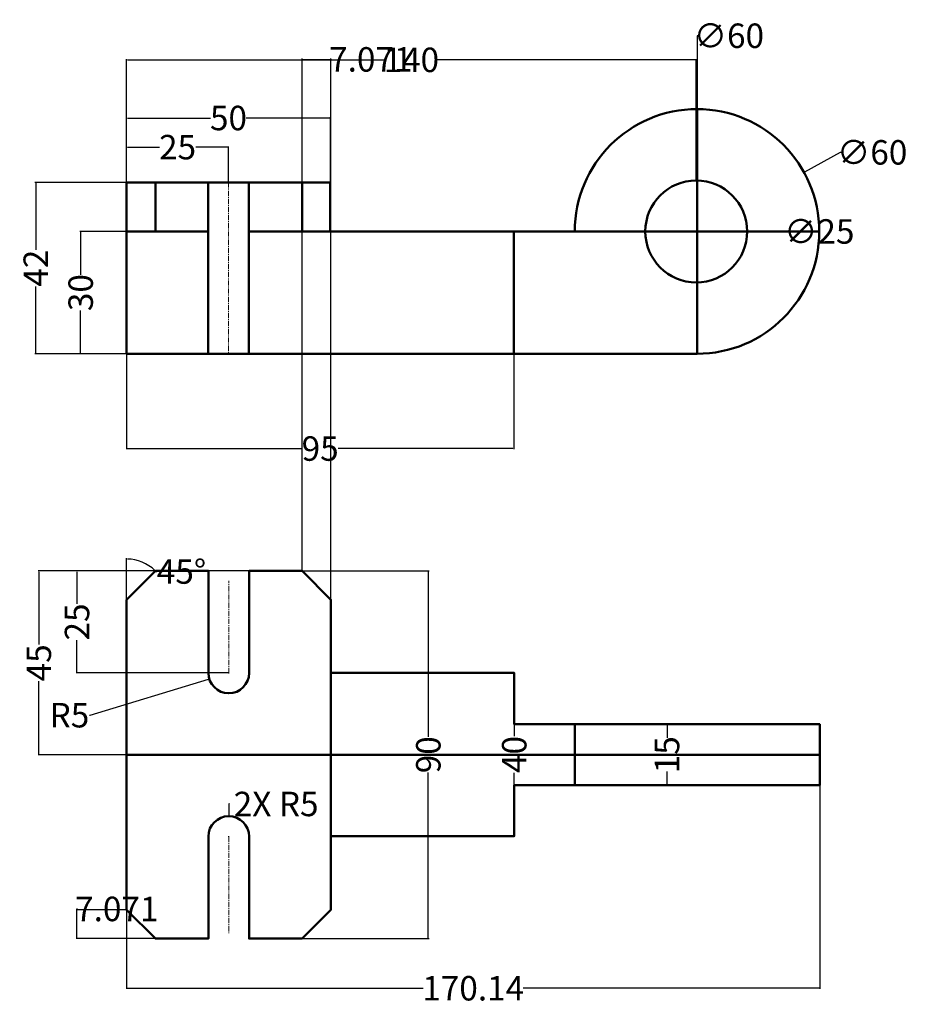
# Model space of a CAD drawing. Units: millimetres. Extents: x 4 to 222, y -16 to 226.
import ezdxf

# ---------------------------------------------------------------- set-up
doc = ezdxf.new("R2010")
doc.units = ezdxf.units.MM
doc.header["$MEASUREMENT"] = 0
doc.linetypes.add('CENTER', pattern=[2, 1.25, -0.25, 0.25, -0.25])
for name, color, linetype, lineweight in [('M-CNTR', 4, 'CENTER', 18), ('M-DIMS', 2, 'Continuous', 25), ('M-OUTL', 7, 'Continuous', 50)]:
    doc.layers.add(name, color=color, linetype=linetype, lineweight=lineweight)
doc.styles.get("Standard").update_dxf_attribs({"font": 'arial.ttf'})
doc.dimstyles.get("Standard").update_dxf_attribs({"dimtxt": 6, "dimasz": 0.18, "dimexe": 0.18, "dimexo": 0.0625, "dimgap": 0.09, "dimtad": 0, "dimtoh": 1, "dimdec": 0, "dimzin": 0, "dimdsep": 46, "dimtxsty": 'Standard', "dimcen": 0.09, "dimadec": 0, "dimazin": 0, "dimtfac": 1, "dimtdec": 0, "dimtofl": 0, "dimtmove": 0, "dimatfit": 3, "dimfxl": 1, "dimtolj": 1, "dimtzin": 0, "dimarcsym": 0})

# ---------------------------------------------------------------- blocks, each defined once
blk = doc.blocks.new('*D1')
at = {"layer": 'Defpoints', "color": 0, "transparency": 16777216}
for p in [(170.41, 216.06), (30.64, 185.97), (170.41, 186.47)]:
    blk.add_point(p, dxfattribs=at)
at = {"layer": 'M-DIMS', "color": 0, "lineweight": -2, "transparency": 16777216}
for p, q in [((30.64, 186.03), (30.64, 216.24)), ((30.82, 216.06), (94.1, 216.06)), ((170.23, 216.06), (106.95, 216.06)), ((170.41, 186.53), (170.41, 216.24))]:
    blk.add_line(p, q, dxfattribs=at)
at = {"layer": 'M-DIMS', "color": 0, "transparency": 16777216}
for points in [[(30.82, 216.09), (30.82, 216.03), (30.64, 216.06)], [(170.23, 216.09), (170.23, 216.03), (170.41, 216.06)]]:
    blk.add_solid(points, dxfattribs=at)
at = {"layer": 'M-DIMS', "color": 0, "transparency": 16777216, "insert": (100.52, 216.06), "char_height": 6, "attachment_point": 5}
blk.add_mtext('\\A1;140', dxfattribs=at)
blk = doc.blocks.new('*D2')
at = {"layer": 'Defpoints', "color": 0, "transparency": 16777216}
for p in [(80.64, 201.79), (30.64, 185.97), (80.64, 185.97)]:
    blk.add_point(p, dxfattribs=at)
at = {"layer": 'M-DIMS', "color": 0, "lineweight": -2, "transparency": 16777216}
for p, q in [((30.64, 186.03), (30.64, 201.97)), ((30.82, 201.79), (51.26, 201.79)), ((80.46, 201.79), (60.02, 201.79)), ((80.64, 186.03), (80.64, 201.97))]:
    blk.add_line(p, q, dxfattribs=at)
at = {"layer": 'M-DIMS', "color": 0, "transparency": 16777216}
for points in [[(30.82, 201.82), (30.82, 201.76), (30.64, 201.79)], [(80.46, 201.82), (80.46, 201.76), (80.64, 201.79)]]:
    blk.add_solid(points, dxfattribs=at)
at = {"layer": 'M-DIMS', "color": 0, "transparency": 16777216, "insert": (55.64, 201.79), "char_height": 6, "attachment_point": 5}
blk.add_mtext('\\A1;50', dxfattribs=at)
blk = doc.blocks.new('*D3')
at = {"layer": 'Defpoints', "color": 0, "transparency": 16777216}
for p in [(55.64, 194.65), (30.64, 185.97), (55.64, 185.97)]:
    blk.add_point(p, dxfattribs=at)
at = {"layer": 'M-DIMS', "color": 0, "lineweight": -2, "transparency": 16777216}
for p, q in [((30.64, 186.03), (30.64, 194.83)), ((30.82, 194.65), (38.68, 194.65)), ((55.46, 194.65), (47.6, 194.65)), ((55.64, 186.03), (55.64, 194.83))]:
    blk.add_line(p, q, dxfattribs=at)
at = {"layer": 'M-DIMS', "color": 0, "transparency": 16777216}
for points in [[(30.82, 194.68), (30.82, 194.62), (30.64, 194.65)], [(55.46, 194.68), (55.46, 194.62), (55.64, 194.65)]]:
    blk.add_solid(points, dxfattribs=at)
at = {"layer": 'M-DIMS', "color": 0, "transparency": 16777216, "insert": (43.14, 194.65), "char_height": 6, "attachment_point": 5}
blk.add_mtext('\\A1;25', dxfattribs=at)
blk = doc.blocks.new('*D4')
at = {"layer": 'Defpoints', "color": 0, "transparency": 16777216}
for p in [(30.64, 185.97), (8.33, 143.97), (30.64, 143.97)]:
    blk.add_point(p, dxfattribs=at)
at = {"layer": 'M-DIMS', "color": 0, "lineweight": -2, "transparency": 16777216}
for p, q in [((30.58, 185.97), (8.15, 185.97)), ((8.33, 185.79), (8.33, 169.45)), ((8.33, 144.15), (8.33, 160.49)), ((30.58, 143.97), (8.15, 143.97))]:
    blk.add_line(p, q, dxfattribs=at)
at = {"layer": 'M-DIMS', "color": 0, "transparency": 16777216}
for points in [[(8.3, 185.79), (8.36, 185.79), (8.33, 185.97)], [(8.3, 144.15), (8.36, 144.15), (8.33, 143.97)]]:
    blk.add_solid(points, dxfattribs=at)
at = {"layer": 'M-DIMS', "color": 0, "transparency": 16777216, "insert": (8.33, 164.97), "char_height": 6, "attachment_point": 5, "rotation": 90}
blk.add_mtext('\\A1;42', dxfattribs=at)
blk = doc.blocks.new('*D5')
at = {"layer": 'Defpoints', "color": 0, "transparency": 16777216}
for p in [(30.64, 173.97), (19.36, 143.97), (30.64, 143.97)]:
    blk.add_point(p, dxfattribs=at)
at = {"layer": 'M-DIMS', "color": 0, "lineweight": -2, "transparency": 16777216}
for p, q in [((30.58, 173.97), (19.18, 173.97)), ((19.36, 173.79), (19.36, 163.34)), ((19.36, 144.15), (19.36, 154.59)), ((30.58, 143.97), (19.18, 143.97))]:
    blk.add_line(p, q, dxfattribs=at)
at = {"layer": 'M-DIMS', "color": 0, "transparency": 16777216}
for points in [[(19.33, 173.79), (19.39, 173.79), (19.36, 173.97)], [(19.33, 144.15), (19.39, 144.15), (19.36, 143.97)]]:
    blk.add_solid(points, dxfattribs=at)
at = {"layer": 'M-DIMS', "color": 0, "transparency": 16777216, "insert": (19.36, 158.97), "char_height": 6, "attachment_point": 5, "rotation": 90}
blk.add_mtext('\\A1;30', dxfattribs=at)
blk = doc.blocks.new('*D6')
at = {"layer": 'Defpoints', "color": 0, "transparency": 16777216}
for p in [(30.64, 143.97), (125.64, 143.97), (125.64, 120.72)]:
    blk.add_point(p, dxfattribs=at)
at = {"layer": 'M-DIMS', "color": 0, "lineweight": -2, "transparency": 16777216}
for p, q in [((30.64, 143.91), (30.64, 120.54)), ((125.64, 143.91), (125.64, 120.54)), ((30.82, 120.72), (73.73, 120.72)), ((125.46, 120.72), (82.55, 120.72))]:
    blk.add_line(p, q, dxfattribs=at)
at = {"layer": 'M-DIMS', "color": 0, "transparency": 16777216}
for points in [[(30.82, 120.75), (30.82, 120.69), (30.64, 120.72)], [(125.46, 120.75), (125.46, 120.69), (125.64, 120.72)]]:
    blk.add_solid(points, dxfattribs=at)
at = {"layer": 'M-DIMS', "color": 0, "transparency": 16777216, "insert": (78.14, 120.72), "char_height": 6, "attachment_point": 5}
blk.add_mtext('\\A1;95', dxfattribs=at)
blk = doc.blocks.new('*D7')
at = {"layer": 'Defpoints', "color": 0, "transparency": 16777216}
for p in [(157.95, 173.97), (182.95, 173.97)]:
    blk.add_point(p, dxfattribs=at)
at = {"layer": 'M-DIMS', "color": 0, "lineweight": -2, "transparency": 16777216}
for p, q in [((170.36, 173.97), (170.54, 173.97)), ((170.45, 173.88), (170.45, 174.06)), ((192.97, 173.97), (183.13, 173.97))]:
    blk.add_line(p, q, dxfattribs=at)
at = {"layer": 'M-DIMS', "color": 0, "transparency": 16777216}
blk.add_solid([(183.13, 174), (183.13, 173.94), (182.95, 173.97)], dxfattribs=at)
at = {"layer": 'M-DIMS', "color": 0, "transparency": 16777216, "insert": (200.64, 173.97), "char_height": 6, "attachment_point": 5}
blk.add_mtext('\\A1;∅25', dxfattribs=at)
blk = doc.blocks.new('*D8')
at = {"layer": 'Defpoints', "color": 0, "transparency": 16777216}
for p in [(196.9, 188.46), (144.37, 159.47)]:
    blk.add_point(p, dxfattribs=at)
at = {"layer": 'M-DIMS', "color": 0, "lineweight": -2, "transparency": 16777216}
for p, q in [((205.8, 193.37), (197.06, 188.55)), ((205.98, 193.37), (205.8, 193.37)), ((170.55, 173.97), (170.73, 173.97)), ((170.64, 173.88), (170.64, 174.06))]:
    blk.add_line(p, q, dxfattribs=at)
at = {"layer": 'M-DIMS', "color": 0, "transparency": 16777216}
blk.add_solid([(197.05, 188.58), (197.08, 188.53), (196.9, 188.46)], dxfattribs=at)
at = {"layer": 'M-DIMS', "color": 0, "transparency": 16777216, "insert": (213.62, 193.37), "char_height": 6, "attachment_point": 5}
blk.add_mtext('\\A1;∅60', dxfattribs=at)
blk = doc.blocks.new('*D9')
at = {"layer": 'Defpoints', "color": 0, "transparency": 16777216}
for p in [(33.23, 93.28), (37.71, 90.69), (30.64, 83.62), (30.64, 83.62), (30.64, 45.62)]:
    blk.add_point(p, dxfattribs=at)
at = {"layer": 'M-DIMS', "color": 0, "lineweight": -2, "transparency": 16777216}
for p, q in [((30.64, 83.68), (30.64, 93.8)), ((37.84, 90.56), (38.02, 90.56))]:
    blk.add_line(p, q, dxfattribs=at)
for start, end in [(46.0313, 88.9687), (43.9687, 45)]:
    blk.add_arc((30.64, 83.62), 10, start, end, dxfattribs=at)
at = {"layer": 'M-DIMS', "color": 0, "transparency": 16777216}
for points in [[(30.82, 93.59), (30.82, 93.65), (30.64, 93.62)], [(37.6, 90.84), (37.56, 90.8), (37.71, 90.69)]]:
    blk.add_solid(points, dxfattribs=at)
at = {"layer": 'M-DIMS', "color": 0, "transparency": 16777216, "insert": (44.11, 90.56), "char_height": 6, "attachment_point": 5}
blk.add_mtext('\\A1;45°', dxfattribs=at)
blk = doc.blocks.new('*D10')
at = {"layer": 'Defpoints', "color": 0, "transparency": 16777216}
for p in [(60.71, 90.69), (9.09, 45.62), (60.71, 45.62)]:
    blk.add_point(p, dxfattribs=at)
at = {"layer": 'M-DIMS', "color": 0, "lineweight": -2, "transparency": 16777216}
for p, q in [((60.65, 90.69), (8.91, 90.69)), ((9.09, 90.51), (9.09, 72.69)), ((9.09, 45.8), (9.09, 63.63)), ((60.65, 45.62), (8.91, 45.62))]:
    blk.add_line(p, q, dxfattribs=at)
at = {"layer": 'M-DIMS', "color": 0, "transparency": 16777216}
for points in [[(9.06, 90.51), (9.12, 90.51), (9.09, 90.69)], [(9.06, 45.8), (9.12, 45.8), (9.09, 45.62)]]:
    blk.add_solid(points, dxfattribs=at)
at = {"layer": 'M-DIMS', "color": 0, "transparency": 16777216, "insert": (9.09, 68.16), "char_height": 6, "attachment_point": 5, "rotation": 90}
blk.add_mtext('\\A1;45', dxfattribs=at)
blk = doc.blocks.new('*D11')
at = {"layer": 'Defpoints', "color": 0, "transparency": 16777216}
for p in [(60.71, 90.69), (18.46, 65.69), (55.71, 65.69)]:
    blk.add_point(p, dxfattribs=at)
at = {"layer": 'M-DIMS', "color": 0, "lineweight": -2, "transparency": 16777216}
for p, q in [((60.65, 90.69), (18.28, 90.69)), ((18.46, 90.51), (18.46, 82.65)), ((18.46, 65.87), (18.46, 73.73)), ((55.65, 65.69), (18.28, 65.69))]:
    blk.add_line(p, q, dxfattribs=at)
at = {"layer": 'M-DIMS', "color": 0, "transparency": 16777216}
for points in [[(18.43, 90.51), (18.49, 90.51), (18.46, 90.69)], [(18.43, 65.87), (18.49, 65.87), (18.46, 65.69)]]:
    blk.add_solid(points, dxfattribs=at)
at = {"layer": 'M-DIMS', "color": 0, "transparency": 16777216, "insert": (18.46, 78.19), "char_height": 6, "attachment_point": 5, "rotation": 90}
blk.add_mtext('\\A1;25', dxfattribs=at)
blk = doc.blocks.new('*D12')
at = {"layer": 'Defpoints', "color": 0, "transparency": 16777216}
for p in [(55.71, 65.69), (50.93, 64.23)]:
    blk.add_point(p, dxfattribs=at)
at = {"layer": 'M-DIMS', "color": 0, "lineweight": -2, "transparency": 16777216}
for p, q in [((55.62, 65.69), (55.8, 65.69)), ((55.71, 65.6), (55.71, 65.78)), ((21.73, 55.32), (50.76, 64.18)), ((21.55, 55.32), (21.73, 55.32))]:
    blk.add_line(p, q, dxfattribs=at)
at = {"layer": 'M-DIMS', "color": 0, "transparency": 16777216}
blk.add_solid([(50.75, 64.21), (50.76, 64.15), (50.93, 64.23)], dxfattribs=at)
at = {"layer": 'M-DIMS', "color": 0, "transparency": 16777216, "insert": (16.6, 55.32), "char_height": 6, "attachment_point": 5}
blk.add_mtext('\\A1;R5', dxfattribs=at)
blk = doc.blocks.new('*D13')
at = {"layer": 'Defpoints', "color": 0, "transparency": 16777216}
for p in [(163.28, 53.12), (163.28, 38.12), (163.28, 38.12)]:
    blk.add_point(p, dxfattribs=at)
at = {"layer": 'M-DIMS', "color": 0, "lineweight": -2, "transparency": 16777216}
for p, q in [((163.28, 52.94), (163.28, 49.75)), ((163.34, 53.12), (163.46, 53.12)), ((163.28, 38.3), (163.28, 41.49)), ((163.34, 38.12), (163.46, 38.12))]:
    blk.add_line(p, q, dxfattribs=at)
at = {"layer": 'M-DIMS', "color": 0, "transparency": 16777216}
for points in [[(163.25, 52.94), (163.31, 52.94), (163.28, 53.12)], [(163.25, 38.3), (163.31, 38.3), (163.28, 38.12)]]:
    blk.add_solid(points, dxfattribs=at)
at = {"layer": 'M-DIMS', "color": 0, "transparency": 16777216, "insert": (163.28, 45.62), "char_height": 6, "attachment_point": 5, "rotation": 90}
blk.add_mtext('\\A1;15', dxfattribs=at)
blk = doc.blocks.new('*D14')
at = {"layer": 'Defpoints', "color": 0, "transparency": 16777216}
for p in [(60.71, 90.69), (60.71, 0.55), (104.69, 0.55)]:
    blk.add_point(p, dxfattribs=at)
at = {"layer": 'M-DIMS', "color": 0, "lineweight": -2, "transparency": 16777216}
for p, q in [((60.77, 90.69), (104.87, 90.69)), ((104.69, 90.51), (104.69, 50)), ((104.69, 0.73), (104.69, 41.24)), ((60.77, 0.55), (104.87, 0.55))]:
    blk.add_line(p, q, dxfattribs=at)
at = {"layer": 'M-DIMS', "color": 0, "transparency": 16777216}
for points in [[(104.66, 90.51), (104.72, 90.51), (104.69, 90.69)], [(104.66, 0.73), (104.72, 0.73), (104.69, 0.55)]]:
    blk.add_solid(points, dxfattribs=at)
at = {"layer": 'M-DIMS', "color": 0, "transparency": 16777216, "insert": (104.69, 45.62), "char_height": 6, "attachment_point": 5, "rotation": 90}
blk.add_mtext('\\A1;90', dxfattribs=at)
blk = doc.blocks.new('*D15')
at = {"layer": 'Defpoints', "color": 0, "transparency": 16777216}
for p in [(103.28, 65.69), (103.28, 25.69), (125.78, 25.69)]:
    blk.add_point(p, dxfattribs=at)
at = {"layer": 'M-DIMS', "color": 0, "lineweight": -2, "transparency": 16777216}
for p, q in [((103.34, 65.69), (125.96, 65.69)), ((125.78, 65.51), (125.78, 50.19)), ((125.78, 25.87), (125.78, 41.19)), ((103.34, 25.69), (125.96, 25.69))]:
    blk.add_line(p, q, dxfattribs=at)
at = {"layer": 'M-DIMS', "color": 0, "transparency": 16777216}
for points in [[(125.75, 65.51), (125.81, 65.51), (125.78, 65.69)], [(125.75, 25.87), (125.81, 25.87), (125.78, 25.69)]]:
    blk.add_solid(points, dxfattribs=at)
at = {"layer": 'M-DIMS', "color": 0, "transparency": 16777216, "insert": (125.78, 45.69), "char_height": 6, "attachment_point": 5, "rotation": 90}
blk.add_mtext('\\A1;40', dxfattribs=at)
blk = doc.blocks.new('*D16')
at = {"layer": 'Defpoints', "color": 0, "transparency": 16777216}
for p in [(80.78, 216.17), (73.71, 90.69), (80.78, 83.62)]:
    blk.add_point(p, dxfattribs=at)
at = {"layer": 'M-DIMS', "color": 0, "lineweight": -2, "transparency": 16777216}
for p, q in [((73.71, 90.75), (73.71, 216.35)), ((73.89, 216.17), (80.6, 216.17)), ((80.78, 83.68), (80.78, 216.35)), ((80.78, 216.17), (80.96, 216.17))]:
    blk.add_line(p, q, dxfattribs=at)
at = {"layer": 'M-DIMS', "color": 0, "transparency": 16777216}
for points in [[(73.89, 216.2), (73.89, 216.14), (73.71, 216.17)], [(80.6, 216.2), (80.6, 216.14), (80.78, 216.17)]]:
    blk.add_solid(points, dxfattribs=at)
at = {"layer": 'M-DIMS', "color": 0, "transparency": 16777216, "insert": (90.57, 216.17), "char_height": 6, "attachment_point": 5}
blk.add_mtext('\\A1;7.071', dxfattribs=at)
blk = doc.blocks.new('*D17')
at = {"layer": 'Defpoints', "color": 0, "transparency": 16777216}
for p in [(18.44, 7.62), (30.64, 7.62), (37.71, 0.55)]:
    blk.add_point(p, dxfattribs=at)
at = {"layer": 'M-DIMS', "color": 0, "lineweight": -2, "transparency": 16777216}
for p, q in [((30.58, 7.62), (18.26, 7.62)), ((18.44, 7.62), (18.44, 7.8)), ((18.44, 7.8), (18.62, 7.8)), ((18.44, 0.73), (18.44, 7.44)), ((37.65, 0.55), (18.26, 0.55))]:
    blk.add_line(p, q, dxfattribs=at)
at = {"layer": 'M-DIMS', "color": 0, "transparency": 16777216}
for points in [[(18.41, 7.44), (18.47, 7.44), (18.44, 7.62)], [(18.41, 0.73), (18.47, 0.73), (18.44, 0.55)]]:
    blk.add_solid(points, dxfattribs=at)
at = {"layer": 'M-DIMS', "color": 0, "transparency": 16777216, "insert": (28.23, 7.8), "char_height": 6, "attachment_point": 5}
blk.add_mtext('\\A1;7.071', dxfattribs=at)
blk = doc.blocks.new('*D18')
at = {"layer": 'Defpoints', "color": 0, "transparency": 16777216}
for p in [(200.78, 38.12), (30.64, 7.62), (200.78, -11.65)]:
    blk.add_point(p, dxfattribs=at)
at = {"layer": 'M-DIMS', "color": 0, "lineweight": -2, "transparency": 16777216}
for p, q in [((200.78, 38.06), (200.78, -11.83)), ((30.64, 7.56), (30.64, -11.83)), ((30.82, -11.65), (103.46, -11.65)), ((200.6, -11.65), (127.96, -11.65))]:
    blk.add_line(p, q, dxfattribs=at)
at = {"layer": 'M-DIMS', "color": 0, "transparency": 16777216}
for points in [[(30.82, -11.62), (30.82, -11.68), (30.64, -11.65)], [(200.6, -11.62), (200.6, -11.68), (200.78, -11.65)]]:
    blk.add_solid(points, dxfattribs=at)
at = {"layer": 'M-DIMS', "color": 0, "transparency": 16777216, "insert": (115.71, -11.65), "char_height": 6, "attachment_point": 5}
blk.add_mtext('\\A1;170.14', dxfattribs=at)
blk = doc.blocks.new('*D19')
at = {"layer": 'Defpoints', "color": 0, "transparency": 16777216}
for p in [(170.64, 203.97), (170.64, 143.97)]:
    blk.add_point(p, dxfattribs=at)
at = {"layer": 'M-DIMS', "color": 0, "lineweight": -2, "transparency": 16777216}
for p, q in [((170.82, 221.97), (170.64, 221.97)), ((170.64, 221.97), (170.64, 204.15)), ((170.55, 173.97), (170.73, 173.97)), ((170.64, 173.88), (170.64, 174.06))]:
    blk.add_line(p, q, dxfattribs=at)
at = {"layer": 'M-DIMS', "color": 0, "transparency": 16777216}
blk.add_solid([(170.61, 204.15), (170.67, 204.15), (170.64, 203.97)], dxfattribs=at)
at = {"layer": 'M-DIMS', "color": 0, "transparency": 16777216, "insert": (178.46, 221.97), "char_height": 6, "attachment_point": 5}
blk.add_mtext('\\A1;∅60', dxfattribs=at)
blk = doc.blocks.new('*D20')
at = {"layer": 'Defpoints', "color": 0, "transparency": 16777216}
for p in [(55.71, 30.55), (55.71, 25.55)]:
    blk.add_point(p, dxfattribs=at)
at = {"layer": 'M-DIMS', "color": 0, "lineweight": -2, "transparency": 16777216}
for p, q in [((55.89, 33.55), (55.71, 33.55)), ((55.71, 33.55), (55.71, 30.73)), ((55.62, 25.55), (55.8, 25.55)), ((55.71, 25.46), (55.71, 25.64))]:
    blk.add_line(p, q, dxfattribs=at)
at = {"layer": 'M-DIMS', "color": 0, "transparency": 16777216}
blk.add_solid([(55.68, 30.73), (55.74, 30.73), (55.71, 30.55)], dxfattribs=at)
at = {"layer": 'M-DIMS', "color": 0, "transparency": 16777216, "insert": (67.34, 33.55), "char_height": 6, "attachment_point": 5}
blk.add_mtext('\\A1;2X R5', dxfattribs=at)

msp = doc.modelspace()

# ---------------------------------------------------------------- linework, layer by layer
at = {"layer": 'M-CNTR'}
for p, q in [((55.6389, 185.9694), (55.6389, 143.9694)), ((55.71, 65.6914), (55.71, 88.2848)), ((55.71, 25.5493), (55.71, 1.8745))]:
    msp.add_line(p, q, dxfattribs=at)
at = {"layer": 'M-OUTL'}
for p, q in [((37.71, 173.9694), (37.71, 185.9694)), ((50.6389, 143.9694), (50.6389, 185.9694)), ((60.6389, 143.9694), (60.6389, 185.9694)), ((73.71, 173.9694), (73.71, 185.9694)), ((140.6389, 173.9694), (60.6389, 173.9694)), ((140.6389, 53.1204), (140.6389, 38.1204))]:
    msp.add_line(p, q, dxfattribs=at)
for points in [[(170.6389, 203.9694), (170.6389, 143.9694), (125.6389, 143.9694), (125.6389, 173.9694)], [(50.6389, 173.9694), (30.6389, 173.9694), (30.6389, 185.9694), (80.6389, 185.9694), (80.6389, 173.9694)], [(125.6389, 143.9694), (30.6389, 143.9694), (30.6389, 173.9694)], [(80.781, 65.6914), (125.781, 65.6914), (125.781, 53.1204), (200.781, 53.1204), (200.781, 38.1204), (125.781, 38.1204), (125.781, 25.6914), (80.781, 25.6914)]]:
    msp.add_lwpolyline(points, dxfattribs=at)
for points in [[(170.6389, 143.9694, 2.41421356), (140.6389, 173.9694), (200.6389, 173.9694)], [(200.781, 45.6204), (30.6389, 45.6204), (30.6389, 83.6204), (37.71, 90.6914), (50.71, 90.6914), (50.71, 65.6914, 1), (60.71, 65.6914), (60.71, 90.6914), (73.71, 90.6914), (80.781, 83.6204), (80.781, 45.6204), (80.781, 7.6204), (73.71, 0.5493), (60.71, 0.5493), (60.71, 25.5493, 1), (50.71, 25.5493), (50.71, 0.5493), (37.71, 0.5493), (30.6389, 7.6204), (30.6389, 45.6204)]]:
    msp.add_lwpolyline(points, format="xyb", dxfattribs=at)
msp.add_circle((170.4503, 173.9694), 12.5, dxfattribs=at)

# ---------------------------------------------------------------- dimensions: what is measured, and where the dimension line sits
at = {"layer": 'M-DIMS'}
for p1, p2, override, picture, middle in [((170.6378, 143.9694), (170.64, 203.9694), {"dimdec": 0, "dimlfac": 1, "dimrnd": 0, "dimzin": 0, "dimdsep": 46, "dimlunit": 2}, '*D19', (178.4618, 221.9694)), ((144.3731, 159.4743), (196.9047, 188.4644), {"dimclrd": 0, "dimclre": 0, "dimclrt": 0}, '*D8', (213.6224, 193.374)), ((157.9503, 173.9694), (182.9503, 173.9694), {"dimclrd": 0, "dimclre": 0, "dimclrt": 0}, '*D7', (200.6389, 173.9694))]:
    dim = msp.add_diameter_dim_2p(p1=p1, p2=p2, dimstyle='Standard', override=override, dxfattribs=at)
    dim.commit()
    dim.dimension.update_dxf_attribs({"geometry": picture, "text_midpoint": middle, "dimtype": 163})
for base, p1, p2, override, picture, middle in [((170.4056, 216.055), (30.6389, 185.9694), (170.4056, 186.4693), {"dimclrd": 0, "dimclre": 0, "dimclrt": 0}, '*D1', (100.5222, 216.055)), ((80.781, 216.1694), (73.71, 90.6914), (80.781, 83.6204), {"dimdec": 3, "dimlfac": 1, "dimrnd": 0, "dimzin": 0, "dimdsep": 46, "dimlunit": 2}, '*D16', (90.5708, 216.1694)), ((80.6389, 201.7872), (30.6389, 185.9694), (80.6389, 185.9694), {"dimclrd": 0, "dimclre": 0, "dimclrt": 0}, '*D2', (55.6389, 201.7872)), ((55.6389, 194.6533), (30.6389, 185.9694), (55.6389, 185.9694), {"dimclrd": 0, "dimclre": 0, "dimclrt": 0}, '*D3', (43.1389, 194.6533)), ((125.6389, 120.7199), (30.6389, 143.9694), (125.6389, 143.9694), {"dimclrd": 0, "dimclre": 0, "dimclrt": 0}, '*D6', (78.1389, 120.7199)), ((200.781, -11.6507), (30.6389, 7.6204), (200.781, 38.1204), {"dimdec": 2, "dimlfac": 1, "dimrnd": 0, "dimzin": 0, "dimdsep": 46, "dimlunit": 2}, '*D18', (115.71, -11.6507))]:
    dim = msp.add_linear_dim(base=base, p1=p1, p2=p2, dimstyle='Standard', override=override, dxfattribs=at)
    dim.commit()
    dim.dimension.update_dxf_attribs({"geometry": picture, "text_midpoint": middle})
for base, p1, p2, override, picture, middle in [((8.3285, 143.9694), (30.6389, 185.9694), (30.6389, 143.9694), {"dimclrd": 0, "dimclre": 0, "dimclrt": 0}, '*D4', (8.3285, 164.9694)), ((19.3624, 143.9694), (30.6389, 173.9694), (30.6389, 143.9694), {"dimclrd": 0, "dimclre": 0, "dimclrt": 0}, '*D5', (19.3624, 158.9694)), ((9.0851, 45.6204), (60.71, 90.6914), (60.71, 45.6204), {"dimclrd": 0, "dimclre": 0, "dimclrt": 0}, '*D10', (9.0851, 68.1559)), ((18.464, 65.6914), (60.71, 90.6914), (55.71, 65.6914), {"dimclrd": 0, "dimclre": 0, "dimclrt": 0}, '*D11', (18.464, 78.1914)), ((104.6907, 0.5493), (60.71, 90.6914), (60.71, 0.5493), {"dimclrd": 0, "dimclre": 0, "dimclrt": 0}, '*D14', (104.6907, 45.6204)), ((125.781, 25.6914), (103.281, 65.6914), (103.281, 25.6914), {"dimclrd": 0, "dimclre": 0, "dimclrt": 0}, '*D15', (125.781, 45.6914)), ((163.281, 38.1204), (163.281, 53.1204), (163.281, 38.1204), {"dimclrd": 0, "dimclre": 0, "dimclrt": 0}, '*D13', (163.281, 45.6204)), ((18.4389, 7.6204), (37.71, 0.5493), (30.6389, 7.6204), {"dimdec": 3, "dimlfac": 1, "dimrnd": 0, "dimzin": 0, "dimdsep": 46, "dimlunit": 2}, '*D17', (28.2287, 7.8004))]:
    dim = msp.add_linear_dim(base=base, p1=p1, p2=p2, angle=90, dimstyle='Standard', override=override, dxfattribs=at)
    dim.commit()
    dim.dimension.update_dxf_attribs({"geometry": picture, "text_midpoint": middle})
dim = msp.add_angular_dim_2l(base=(33.2271, 93.2796), line1=((30.6389, 45.6204), (30.6389, 83.6204)), line2=((30.6389, 83.6204), (37.71, 90.6914)), dimstyle='Standard', override={"dimclrd": 0, "dimclre": 0, "dimclrt": 0}, dxfattribs=at)
dim.commit()
dim.dimension.update_dxf_attribs({"geometry": '*D9', "text_midpoint": (44.1122, 90.563)})
dim = msp.add_radius_dim(center=(55.71, 65.6914), mpoint=(50.9279, 64.2313), dimstyle='Standard', override={"dimclrd": 0, "dimclre": 0, "dimclrt": 0}, dxfattribs=at)
dim.commit()
dim.dimension.update_dxf_attribs({"geometry": '*D12', "text_midpoint": (16.5961, 55.3153), "dimtype": 164})
dim = msp.add_radius_dim(center=(55.71, 25.5493), mpoint=(55.71, 30.5493), text='2X <>', dimstyle='Standard', override={"dimdec": 0, "dimlfac": 1, "dimrnd": 0, "dimzin": 0, "dimdsep": 46, "dimlunit": 2}, dxfattribs=at)
dim.commit()
dim.dimension.update_dxf_attribs({"geometry": '*D20', "text_midpoint": (67.3375, 33.5493), "dimtype": 164})

doc.saveas('drawing.dxf')
